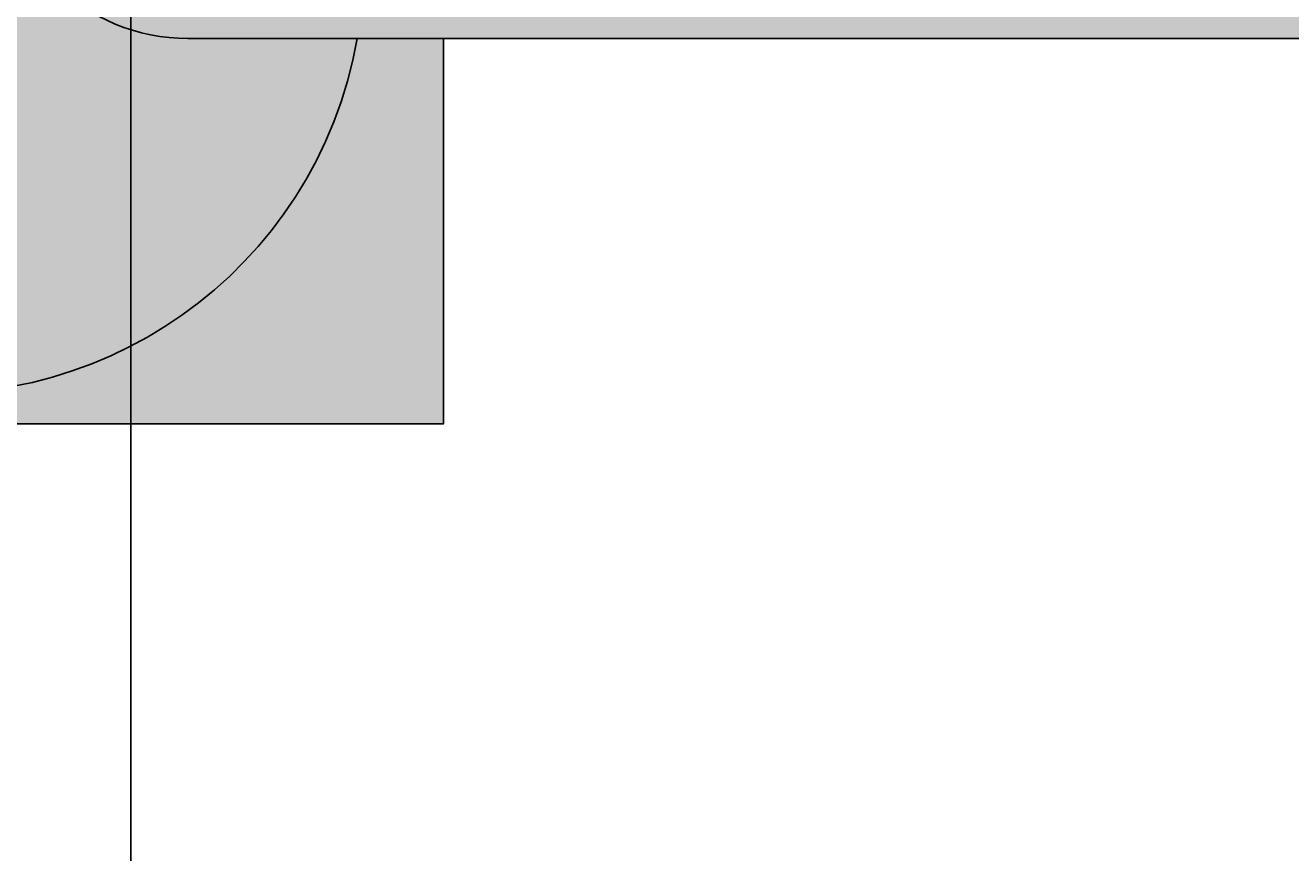
# Model space of a CAD drawing. Units: millimetres. Extents: x -11 to 280, y -4 to 208.
# Tile 32 of 55: x 189 to 222, y 54 to 76. Entities that reach past the tile are written whole.
import ezdxf

# ---------------------------------------------------------------- set-up
doc = ezdxf.new("R2010")
doc.units = ezdxf.units.MM
for name, color, linetype, lineweight in [('M-DIMS', 2, 'Continuous', 18), ('M-HYDR-PRES', 7, 'Continuous', 25), ('M-HYDR-VALV', 7, 'Continuous', 25), ('M-HYDR-VALV-PATT', 252, 'Continuous', 13)]:
    doc.layers.add(name, color=color, linetype=linetype, lineweight=lineweight)
doc.layers.add('M-HYDR-PRES-PATT', color=240, linetype='Continuous', lineweight=13, true_color=0xed1f24)
doc.styles.get("Standard").update_dxf_attribs({"font": 'arial.ttf'})
doc.dimstyles.get("Standard").update_dxf_attribs({"dimtxt": 0.18, "dimasz": 0.18, "dimexe": 0.18, "dimexo": 0.0625, "dimgap": 0.09, "dimtad": 0, "dimtih": 1, "dimtoh": 1, "dimdec": 4, "dimzin": 0, "dimdsep": 46, "dimtxsty": 'Standard', "dimcen": 0.09, "dimadec": 0, "dimazin": 0, "dimtfac": 1, "dimtdec": 4, "dimtofl": 0, "dimtmove": 0, "dimatfit": 3, "dimfxl": 1, "dimtolj": 1, "dimtzin": 0, "dimarcsym": 0})

# ---------------------------------------------------------------- blocks, each defined once
blk = doc.blocks.new('*D4')
at = {"layer": 'Defpoints', "color": 0, "transparency": 16777216}
for p in [(4.763, 84.426), (266.035, 51.733), (266.035, -3.415)]:
    blk.add_point(p, dxfattribs=at)
at = {"layer": 'M-DIMS', "color": 0, "lineweight": -2, "transparency": 16777216}
for p, q in [((4.763, 84.364), (4.763, -3.595)), ((266.035, 51.67), (266.035, -3.595)), ((4.943, -3.415), (134.934, -3.415)), ((265.855, -3.415), (135.864, -3.415))]:
    blk.add_line(p, q, dxfattribs=at)
at = {"layer": 'M-DIMS', "color": 0, "transparency": 16777216}
for points in [[(4.943, -3.385), (4.943, -3.445), (4.763, -3.415)], [(265.855, -3.385), (265.855, -3.445), (266.035, -3.415)]]:
    blk.add_solid(points, dxfattribs=at)
at = {"layer": 'M-DIMS', "color": 0, "transparency": 16777216, "insert": (135.399, -3.415), "char_height": 0.18, "attachment_point": 5}
blk.add_mtext('\\A1;261.27', dxfattribs=at)
blk = doc.blocks.new('*D5')
at = {"layer": 'Defpoints', "color": 0, "transparency": 16777216}
for p in [(24.759, 192.645), (-10.087, 11.435), (261.686, 11.435)]:
    blk.add_point(p, dxfattribs=at)
at = {"layer": 'M-DIMS', "color": 0, "lineweight": -2, "transparency": 16777216}
for p, q in [((24.696, 192.645), (-10.267, 192.645)), ((-10.087, 192.465), (-10.087, 102.222)), ((-10.087, 11.615), (-10.087, 101.858)), ((261.624, 11.435), (-10.267, 11.435))]:
    blk.add_line(p, q, dxfattribs=at)
at = {"layer": 'M-DIMS', "color": 0, "transparency": 16777216}
for points in [[(-10.117, 192.465), (-10.057, 192.465), (-10.087, 192.645)], [(-10.117, 11.615), (-10.057, 11.615), (-10.087, 11.435)]]:
    blk.add_solid(points, dxfattribs=at)
at = {"layer": 'M-DIMS', "color": 0, "transparency": 16777216, "insert": (-10.087, 102.04), "char_height": 0.18, "attachment_point": 5}
blk.add_mtext('\\A1;181.2', dxfattribs=at)
blk = doc.blocks.new('*D13')
at = {"layer": 'Defpoints', "color": 0, "transparency": 16777216}
for p in [(191.774, 105.314), (232.2, 105.314), (232.2, -3.415)]:
    blk.add_point(p, dxfattribs=at)
at = {"layer": 'M-DIMS', "color": 0, "lineweight": -2, "transparency": 16777216}
for p, q in [((191.774, 105.252), (191.774, -3.595)), ((232.2, 105.252), (232.2, -3.595)), ((191.954, -3.415), (211.52, -3.415)), ((232.02, -3.415), (212.454, -3.415))]:
    blk.add_line(p, q, dxfattribs=at)
at = {"layer": 'M-DIMS', "color": 0, "transparency": 16777216}
for points in [[(191.954, -3.385), (191.954, -3.445), (191.774, -3.415)], [(232.02, -3.385), (232.02, -3.445), (232.2, -3.415)]]:
    blk.add_solid(points, dxfattribs=at)
at = {"layer": 'M-DIMS', "color": 0, "transparency": 16777216, "insert": (211.987, -3.415), "char_height": 0.18, "attachment_point": 5}
blk.add_mtext('\\A1;40.426', dxfattribs=at)
blk = doc.blocks.new('*D20')
at = {"layer": 'Defpoints', "color": 0, "transparency": 16777216}
for p in [(231.68, 207.495), (151.022, 43.599), (231.68, 43.599)]:
    blk.add_point(p, dxfattribs=at)
at = {"layer": 'M-DIMS', "color": 0, "lineweight": -2, "transparency": 16777216}
for p, q in [((151.022, 43.662), (151.022, 207.675)), ((231.68, 43.662), (231.68, 207.675)), ((151.202, 207.495), (190.957, 207.495)), ((231.5, 207.495), (191.745, 207.495))]:
    blk.add_line(p, q, dxfattribs=at)
at = {"layer": 'M-DIMS', "color": 0, "transparency": 16777216}
for points in [[(151.202, 207.525), (151.202, 207.465), (151.022, 207.495)], [(231.5, 207.525), (231.5, 207.465), (231.68, 207.495)]]:
    blk.add_solid(points, dxfattribs=at)
at = {"layer": 'M-DIMS', "color": 0, "transparency": 16777216, "insert": (191.351, 207.495), "char_height": 0.18, "attachment_point": 5}
blk.add_mtext('\\A1;80.66', dxfattribs=at)

msp = doc.modelspace()

# ---------------------------------------------------------------- hatches: boundary and pattern name
at = {"layer": 'M-HYDR-PRES-PATT'}
h = msp.add_hatch(color=256, dxfattribs=at)
h.set_gradient(color1=(237, 31, 36), color2=(237, 31, 36), tint=1)
h.paths.add_polyline_path([(232.2, 133.1228), (228.7, 133.1228), (228.7, 108.8141), (102.7646, 108.8141), (102.7646, 105.3141), (232.2, 105.3141)])
h.paths.add_polyline_path([(128.8433, 105.3141), (125.3433, 105.3141), (125.3433, 91.7099, 1), (128.8433, 91.7099)])
h.paths.add_polyline_path([(229.1617, 78.7098), (196.7745, 78.7098, -0.4142136), (191.7745, 83.7098), (191.7745, 105.3141), (188.2745, 105.3141), (188.2745, 80.2098, 0.4142136), (193.2745, 75.2098), (225.6617, 75.2098), (225.6617, 43.5991), (229.1617, 43.5991)])
h.paths.add_polyline_path([(102.7646, 110.3704), (95.5776, 110.3704), (95.5776, 103.9022), (102.7646, 103.9022)])
h.paths.add_polyline_path([(100.7059, 107.2502), (99.1711, 106.3641), (99.1711, 106.8641), (97.1711, 106.8641), (97.1711, 107.6363), (99.1711, 107.6363), (99.1711, 108.1363)], flags=16)
h.paths.add_polyline_path([(234.6119, 138.4081), (226.5106, 138.4081), (226.5106, 133.1228), (234.6119, 133.1228)])
h.paths.add_polyline_path([(231.1963, 135.7055), (230.2965, 134.1786), (229.4241, 135.7213), (229.9241, 135.7168), (229.9418, 137.7167), (230.7141, 137.7099), (230.6963, 135.71)], flags=16)
at = {"layer": 'M-HYDR-VALV-PATT'}
h = msp.add_hatch(color=256, dxfattribs=at)
h.set_gradient(color1=(153, 27, 30), color2=(153, 27, 30), tint=1)
h.paths.add_polyline_path([(131.8437, 88.2421, -0.3394543), (132.5849, 89.208), (121.2548, 86.1721, -0.4931454), (122.5137, 85.2062, -0.3394543), (121.7725, 84.2403), (133.1025, 87.2762, -0.4931454)])
h.paths.add_polyline_path([(133.1025, 83.1351, -0.4931454), (131.8437, 84.101, -0.3394543), (132.5849, 85.0669), (121.2548, 82.031, -0.4931454), (122.5137, 81.0651, -0.3394543), (121.7725, 80.0992)])
h.paths.add_polyline_path([(133.1025, 78.994, -0.4931454), (131.8437, 79.9599, -0.3394543), (132.5849, 80.9258), (121.2548, 77.8899, -0.4931454), (122.5137, 76.924, -0.3394543), (121.7725, 75.9581)])
h.paths.add_polyline_path([(197.7905, 78.7098), (200.0003, 78.7098), (200.0003, 89.3873), (191.7745, 89.3873), (191.7745, 87.1776, -0.2439164)])
h.paths.add_polyline_path([(200.0003, 65.0638), (200.0003, 75.2098), (197.7325, 75.2098, -0.4135811), (184.7092, 66.0277), (184.7092, 65.0638)])
h.paths.add_polyline_path([(181.2092, 65.0638), (181.2092, 67.2471, -0.2598454), (175.3563, 76.54), (173.8038, 76.54), (173.8038, 65.0638)])
h.paths.add_polyline_path([(188.2745, 88.3022), (188.2745, 89.3873), (173.8038, 89.3873), (173.8038, 80.04), (175.7181, 80.04, -0.3816661)])
h = msp.add_hatch(color=256, dxfattribs=at)
h.set_gradient(color1=(205, 105, 40), color2=(34, 52, 110), tint=1, name='INVCYLINDER')
h.paths.add_polyline_path([(188.2745, 80.2098), (188.2745, 88.3022, 0.3816661), (175.7181, 80.04), (179.7092, 80.04, -0.4142136), (184.7092, 75.04), (184.7092, 66.0277, 0.4135811), (197.7325, 75.2098), (193.2745, 75.2098, -0.4142136)])
h.paths.add_polyline_path([(176.2092, 76.54), (175.3563, 76.54, 0.2598454), (181.2092, 67.2471), (181.2092, 71.54, 0.4142136)])
h.paths.add_polyline_path([(196.7745, 78.7098), (197.7905, 78.7098, 0.2439164), (191.7745, 87.1776), (191.7745, 83.7098, 0.4142136)])

# ---------------------------------------------------------------- linework, layer by layer
at = {"layer": 'M-HYDR-PRES'}
msp.add_lwpolyline([(188.2745, 105.3141), (188.2745, 80.2098, 0.4142136), (193.2745, 75.2098), (225.6617, 75.2098), (225.6617, 43.5991)], format="xyb", dxfattribs=at)
at = {"layer": 'M-HYDR-VALV'}
msp.add_lwpolyline([(200.0003, 75.2098), (200.0003, 65.0638), (184.7092, 65.0638)], dxfattribs=at)
msp.add_arc((186.6199, 77.1445), 11.2798, 260.24776, 350.12401, dxfattribs=at)

# ---------------------------------------------------------------- dimensions: what is measured, and where the dimension line sits
at = {"layer": 'M-DIMS'}
for base, p1, p2, override, picture, middle in [((231.6803, 207.495), (151.0217, 43.5991), (231.6803, 43.5991), {"dimdec": 2, "dimlfac": 1, "dimrnd": 0, "dimzin": 0, "dimdsep": 46, "dimlunit": 2}, '*D20', (191.351, 207.495)), ((232.20002, -3.41542), (191.77448, 105.31407), (232.20002, 105.31407), {"dimdec": 3, "dimlfac": 1, "dimrnd": 0, "dimzin": 0, "dimdsep": 46, "dimlunit": 2}, '*D13', (211.98725, -3.41542)), ((266.0352, -3.4154), (4.7635, 84.4261), (266.0352, 51.7328), {"dimdec": 2, "dimlfac": 1, "dimrnd": 0, "dimzin": 0, "dimdsep": 46, "dimlunit": 2}, '*D4', (135.3993, -3.4154))]:
    dim = msp.add_linear_dim(base=base, p1=p1, p2=p2, dimstyle='Standard', override=override, dxfattribs=at)
    dim.commit()
    dim.dimension.update_dxf_attribs({"geometry": picture, "text_midpoint": middle})
dim = msp.add_linear_dim(base=(-10.0865, 11.4346), p1=(24.7588, 192.645), p2=(261.6863, 11.4346), angle=90, dimstyle='Standard', override={"dimdec": 1, "dimlfac": 1, "dimrnd": 0, "dimzin": 0, "dimdsep": 46, "dimlunit": 2}, dxfattribs=at)
dim.commit()
dim.dimension.update_dxf_attribs({"geometry": '*D5', "text_midpoint": (-10.0865, 102.0398)})

doc.saveas('drawing.dxf')
